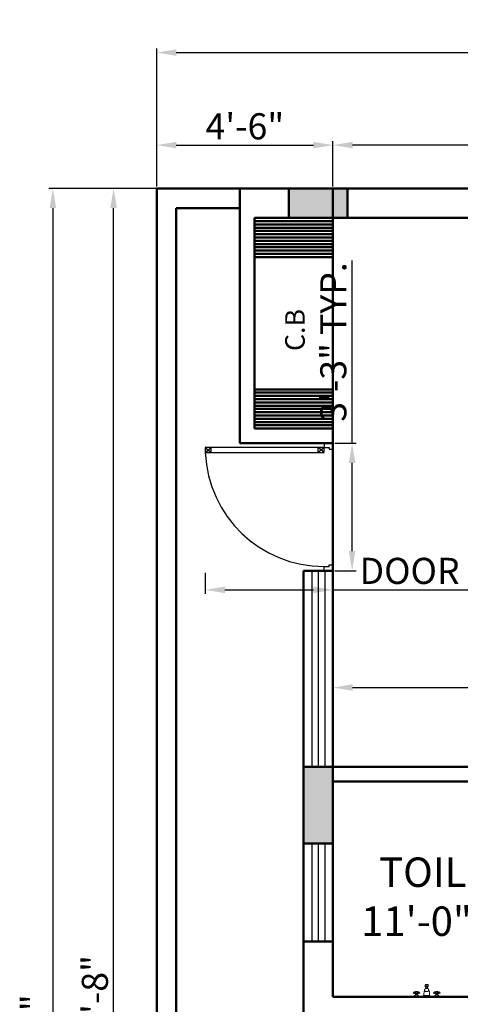
# Model space of a CAD drawing. Units: millimetres. Extents: x 1706 to 5913, y 156 to 1716.
# Tile 14 of 26: x 3136 to 3271, y 1414 to 1716. Entities that reach past the tile are written whole.
import ezdxf

# ---------------------------------------------------------------- set-up
doc = ezdxf.new("R2010")
doc.units = ezdxf.units.MM
for name, color, linetype, lineweight in [('A-ANNO-DIMS', 2, 'Continuous', 18), ('A-AREA-IDEN', 3, 'Continuous', 18), ('A-COLS', 20, 'Continuous', 50), ('A-DOOR', 4, 'Continuous', 25), ('A-FLOR-FIXT', 8, 'Continuous', 18), ('A-GLAZ', 150, 'Continuous', 25), ('A-WALL', 7, 'Continuous', 50)]:
    doc.layers.add(name, color=color, linetype=linetype, lineweight=lineweight)
doc.styles.get("Standard").update_dxf_attribs({"font": 'arial.ttf'})
doc.dimstyles.new('ISO-25', dxfattribs={"dimtxt": 8, "dimasz": 6, "dimexe": 1.25, "dimexo": 0.625, "dimtad": 1, "dimdec": 0, "dimlunit": 3, "dimtxsty": 'Standard', "dimcen": 2.5, "dimadec": 0, "dimazin": 0, "dimtfac": 1, "dimtdec": 0, "dimtmove": 0, "dimatfit": 3, "dimfxl": 1, "dimarcsym": 0})

# ---------------------------------------------------------------- blocks, each defined once
blk = doc.blocks.new('Puerta 01')
for p, q in [((-0.7745, -0.0264), (-0.7368, -0.0584)), ((-0.7745, -0.0584), (-0.7368, -0.0264)), ((-0.7368, -0.0584), (-0.7368, -0.0264)), ((-0.028, -0.0584), (-0.0657, -0.0264)), ((-0.028, -0.0264), (-0.0657, -0.0584)), ((-0.0657, -0.0584), (-0.0657, -0.0264))]:
    blk.add_line(p, q)
for points in [[(-0.028, 0), (-0.028, -0.0264), (0.004, -0.0264), (0.004, -0.036), (0.028, -0.036), (0.028, 0)], [(-0.028, -0.0264), (-0.7745, -0.0264), (-0.7745, -0.0584), (-0.028, -0.0584)], [(0.004, -0.7736), (0.004, -0.764), (0.028, -0.764), (0.028, -0.8), (-0.028, -0.8), (-0.028, -0.7736)]]:
    blk.add_lwpolyline(points, close=True)
blk.add_arc((-0.028, -0.0264), 0.7472, 182.45453, 270)
blk = doc.blocks.new('Faucet - Bathroom front')
for p, q in [((-0.5, 4.25), (0.5, 4.25)), ((0.5, 3.75), (-0.5, 3.75)), ((-5, 0), (-2.25, 0)), ((-4.5087, 0.25), (-2.7408, 0.25)), ((-4, 1.625), (-4.25, 1.625)), ((-4, 1.375), (-4.25, 1.375)), ((-3.1442, 0.75), (-4.0979, 0.75)), ((-3.25, 1.625), (-3, 1.625)), ((-3.25, 1.375), (-3, 1.375)), ((-1.5, 0), (1.5, 0)), ((-1, 0.5), (1, 0.5)), ((-0.5, 3), (0.5, 3)), ((0.5, 2), (-0.5, 2)), ((-0.25, 3), (-0.25, 3.5)), ((0.25, 3.5), (0.25, 3)), ((2.25, 0), (5, 0)), ((2.7413, 0.25), (4.5092, 0.25)), ((3.25, 1.625), (3, 1.625)), ((3.25, 1.375), (3, 1.375)), ((4.1058, 0.75), (3.1521, 0.75)), ((4, 1.625), (4.25, 1.625)), ((4, 1.375), (4.25, 1.375))]:
    blk.add_line(p, q)
for points in [[(-0.5, 3.75), (-0.5, 4.25)], [(-0.25, 4.5), (0.25, 4.5)], [(0.5, 4.25), (0.5, 3.75)], [(0.25, 3.5), (-0.25, 3.5)]]:
    blk.add_lwpolyline(points)
for points in [[(-4, 1), (-4, 2), (-3.25, 2), (-3.25, 1)], [(3.25, 1), (3.25, 2), (4, 2), (4, 1)]]:
    blk.add_lwpolyline(points, close=True)
for centre in [(-4.5, 1.5), (-3.625, 1.5), (-2.75, 1.5), (2.75, 1.5), (3.625, 1.5), (4.5, 1.5)]:
    blk.add_circle(centre, 0.2795)
for centre, radius, start, end in [((-0.2575, 4.2575), 0.2426, 88.22243, 181.7776), ((-0.2575, 3.7425), 0.2426, 178.2224, 271.7776), ((0.2575, 4.2575), 0.2426, 358.2224, 91.77757), ((0.2575, 3.7425), 0.2426, 268.2224, 1.777565), ((-5.375, 1.375), 1.4252, 285.2551, 344.7449), ((-1.875, 1.375), 1.4252, 195.2551, 254.7449), ((-0.7962, -0.2038), 0.7327, 106.1502, 163.8498), ((3, 1), 4.0311, 150.2551, 187.125), ((0.6413, 2.5), 1.246, 156.3417, 203.6583), ((-3, 1), 4.0311, 352.875, 29.74488), ((-0.6413, 2.5), 1.246, 336.3417, 23.65835), ((0.7962, -0.2038), 0.7327, 16.1502, 73.84979), ((1.875, 1.375), 1.4252, 285.2551, 344.7449), ((5.375, 1.375), 1.4252, 195.2551, 254.7449)]:
    blk.add_arc(centre, radius, start, end)
blk = doc.blocks.new('*D48')
at = {"layer": 'A-ANNO-DIMS', "color": 0, "lineweight": -2, "transparency": 16777216}
for p, q in [((3231.71, 1527.55), (3231.71, 1510.16)), ((3512.21, 1527.55), (3512.21, 1510.16)), ((3237.71, 1511.41), (3506.21, 1511.41))]:
    blk.add_line(p, q, dxfattribs=at)
at = {"layer": 'A-ANNO-DIMS', "color": 0, "transparency": 16777216}
for points in [[(3237.71, 1512.41), (3237.71, 1510.41), (3231.71, 1511.41)], [(3506.21, 1512.41), (3506.21, 1510.41), (3512.21, 1511.41)]]:
    blk.add_solid(points, dxfattribs=at)
at = {"layer": 'Defpoints', "color": 0, "transparency": 16777216}
for p in [(3231.71, 1528.17), (3512.21, 1528.17), (3512.21, 1511.41)]:
    blk.add_point(p, dxfattribs=at)
at = {"layer": 'A-ANNO-DIMS', "color": 0, "transparency": 16777216, "insert": (3371.96, 1516.12), "char_height": 8, "attachment_point": 5}
blk.add_mtext('23\'-5"', dxfattribs=at)
blk = doc.blocks.new('*D106')
at = {"layer": 'A-ANNO-DIMS', "color": 0, "lineweight": -2, "transparency": 16777216}
for p, q in [((3177.08, 1664.18), (3144.63, 1664.18)), ((3145.88, 1658.18), (3145.88, 1146.68)), ((3177.08, 1140.68), (3144.63, 1140.68))]:
    blk.add_line(p, q, dxfattribs=at)
at = {"layer": 'A-ANNO-DIMS', "color": 0, "transparency": 16777216}
for points in [[(3144.88, 1658.18), (3146.88, 1658.18), (3145.88, 1664.18)], [(3144.88, 1146.68), (3146.88, 1146.68), (3145.88, 1140.68)]]:
    blk.add_solid(points, dxfattribs=at)
at = {"layer": 'Defpoints', "color": 0, "transparency": 16777216}
for p in [(3177.71, 1664.18), (3145.88, 1140.68), (3177.71, 1140.68)]:
    blk.add_point(p, dxfattribs=at)
at = {"layer": 'A-ANNO-DIMS', "color": 0, "transparency": 16777216, "insert": (3141.17, 1402.43), "char_height": 8, "attachment_point": 5, "rotation": 90}
blk.add_mtext('43\'-8"', dxfattribs=at)
blk = doc.blocks.new('*D107')
at = {"layer": 'A-ANNO-DIMS', "color": 0, "lineweight": -2, "transparency": 16777216}
for p, q in [((3202.58, 1664.18), (3163.24, 1664.18)), ((3164.49, 1170.68), (3164.49, 1658.18)), ((3202.58, 1164.68), (3163.24, 1164.68))]:
    blk.add_line(p, q, dxfattribs=at)
at = {"layer": 'A-ANNO-DIMS', "color": 0, "transparency": 16777216}
for points in [[(3163.49, 1658.18), (3165.49, 1658.18), (3164.49, 1664.18)], [(3163.49, 1170.68), (3165.49, 1170.68), (3164.49, 1164.68)]]:
    blk.add_solid(points, dxfattribs=at)
at = {"layer": 'Defpoints', "color": 0, "transparency": 16777216}
for p in [(3164.49, 1664.18), (3203.21, 1664.18), (3203.21, 1164.68)]:
    blk.add_point(p, dxfattribs=at)
at = {"layer": 'A-ANNO-DIMS', "color": 0, "transparency": 16777216, "insert": (3159.78, 1414.43), "char_height": 8, "attachment_point": 5, "rotation": 90}
blk.add_mtext('41\'-8"', dxfattribs=at)
blk = doc.blocks.new('*D108')
at = {"layer": 'A-ANNO-DIMS', "color": 0, "lineweight": -2, "transparency": 16777216}
for p, q in [((3177.71, 1664.81), (3177.71, 1678.72)), ((3183.71, 1677.47), (3225.71, 1677.47)), ((3231.71, 1664.81), (3231.71, 1678.72))]:
    blk.add_line(p, q, dxfattribs=at)
at = {"layer": 'A-ANNO-DIMS', "color": 0, "transparency": 16777216}
for points in [[(3183.71, 1678.47), (3183.71, 1676.47), (3177.71, 1677.47)], [(3225.71, 1678.47), (3225.71, 1676.47), (3231.71, 1677.47)]]:
    blk.add_solid(points, dxfattribs=at)
at = {"layer": 'Defpoints', "color": 0, "transparency": 16777216}
for p in [(3231.71, 1677.47), (3177.71, 1664.18), (3231.71, 1664.18)]:
    blk.add_point(p, dxfattribs=at)
at = {"layer": 'A-ANNO-DIMS', "color": 0, "transparency": 16777216, "insert": (3204.71, 1682.18), "char_height": 8, "attachment_point": 5}
blk.add_mtext('4\'-6"', dxfattribs=at)
blk = doc.blocks.new('*D109')
at = {"layer": 'A-ANNO-DIMS', "color": 0, "lineweight": -2, "transparency": 16777216}
for p, q in [((3231.71, 1664.81), (3231.71, 1678.72)), ((3927.82, 1677.47), (3237.71, 1677.47)), ((3933.82, 1664.81), (3933.82, 1678.72))]:
    blk.add_line(p, q, dxfattribs=at)
at = {"layer": 'A-ANNO-DIMS', "color": 0, "transparency": 16777216}
for points in [[(3237.71, 1678.47), (3237.71, 1676.47), (3231.71, 1677.47)], [(3927.82, 1678.47), (3927.82, 1676.47), (3933.82, 1677.47)]]:
    blk.add_solid(points, dxfattribs=at)
at = {"layer": 'Defpoints', "color": 0, "transparency": 16777216}
for p in [(3231.71, 1677.47), (3231.71, 1664.18), (3933.82, 1664.18)]:
    blk.add_point(p, dxfattribs=at)
at = {"layer": 'A-ANNO-DIMS', "color": 0, "transparency": 16777216, "insert": (3582.76, 1682.18), "char_height": 8, "attachment_point": 5}
blk.add_mtext('58\'-6"', dxfattribs=at)
blk = doc.blocks.new('*D111')
at = {"layer": 'A-ANNO-DIMS', "color": 0, "lineweight": -2, "transparency": 16777216}
for p, q in [((3177.71, 1664.81), (3177.71, 1707.03)), ((4073, 1664.81), (4073, 1707.03)), ((3183.71, 1705.78), (4067, 1705.78))]:
    blk.add_line(p, q, dxfattribs=at)
at = {"layer": 'A-ANNO-DIMS', "color": 0, "transparency": 16777216}
for points in [[(3183.71, 1706.78), (3183.71, 1704.78), (3177.71, 1705.78)], [(4067, 1706.78), (4067, 1704.78), (4073, 1705.78)]]:
    blk.add_solid(points, dxfattribs=at)
at = {"layer": 'Defpoints', "color": 0, "transparency": 16777216}
for p in [(4073, 1705.78), (3177.71, 1664.18), (4073, 1664.18)]:
    blk.add_point(p, dxfattribs=at)
at = {"layer": 'A-ANNO-DIMS', "color": 0, "transparency": 16777216, "insert": (3625.35, 1710.41), "char_height": 8, "attachment_point": 5}
blk.add_mtext('74\'-7"', dxfattribs=at)
blk = doc.blocks.new('*D211')
at = {"layer": 'A-ANNO-DIMS', "color": 0, "lineweight": -2, "transparency": 16777216}
for p, q in [((3192.58, 1546.56), (3192.58, 1540.06)), ((3231.71, 1546.56), (3231.71, 1540.06)), ((3198.58, 1541.31), (3225.71, 1541.31)), ((3231.71, 1541.31), (3323.96, 1541.31))]:
    blk.add_line(p, q, dxfattribs=at)
at = {"layer": 'A-ANNO-DIMS', "color": 0, "transparency": 16777216}
for points in [[(3198.58, 1542.31), (3198.58, 1540.31), (3192.58, 1541.31)], [(3225.71, 1542.31), (3225.71, 1540.31), (3231.71, 1541.31)]]:
    blk.add_solid(points, dxfattribs=at)
at = {"layer": 'Defpoints', "color": 0, "transparency": 16777216}
for p in [(3192.58, 1547.18), (3231.71, 1547.18), (3231.71, 1541.31)]:
    blk.add_point(p, dxfattribs=at)
at = {"layer": 'A-ANNO-DIMS', "color": 0, "transparency": 16777216, "insert": (3280.83, 1546.08), "char_height": 8, "attachment_point": 5}
blk.add_mtext('DOOR 3\'-3" TYP.', dxfattribs=at)
blk = doc.blocks.new('*D212')
at = {"layer": 'A-ANNO-DIMS', "color": 0, "lineweight": -2, "transparency": 16777216}
for p, q in [((3237.58, 1586.18), (3237.58, 1642.19)), ((3232.33, 1586.18), (3238.83, 1586.18)), ((3237.58, 1553.18), (3237.58, 1580.18)), ((3232.33, 1547.18), (3238.83, 1547.18))]:
    blk.add_line(p, q, dxfattribs=at)
at = {"layer": 'A-ANNO-DIMS', "color": 0, "transparency": 16777216}
for points in [[(3236.58, 1580.18), (3238.58, 1580.18), (3237.58, 1586.18)], [(3236.58, 1553.18), (3238.58, 1553.18), (3237.58, 1547.18)]]:
    blk.add_solid(points, dxfattribs=at)
at = {"layer": 'Defpoints', "color": 0, "transparency": 16777216}
for p in [(3231.71, 1586.18), (3237.58, 1586.18), (3231.71, 1547.18)]:
    blk.add_point(p, dxfattribs=at)
at = {"layer": 'A-ANNO-DIMS', "color": 0, "transparency": 16777216, "insert": (3232.86, 1617.18), "char_height": 8, "attachment_point": 5, "rotation": 90}
blk.add_mtext('3\'-3" TYP.', dxfattribs=at)

msp = doc.modelspace()

# ---------------------------------------------------------------- hatches: boundary and pattern name
at = {"layer": 'A-COLS'}
h = msp.add_hatch(color=256, dxfattribs=at)
h.dxf.hatch_style = 1
h.paths.add_polyline_path([(3236.21, 1664.18), (3218.21, 1664.18), (3218.21, 1655.18), (3236.21, 1655.18)])
h = msp.add_hatch(color=256, dxfattribs=at)
h.dxf.hatch_style = 1
h.paths.add_polyline_path([(3231.71, 1487.18), (3222.71, 1487.18), (3222.71, 1463.68), (3231.71, 1463.68)])

# ---------------------------------------------------------------- linework, layer by layer
msp.add_lwpolyline([(3236.43, 1664.18), (3218.21, 1664.18), (3218.21, 1655.18), (3236.21, 1655.18), (3236.21, 1664.18)], dxfattribs=at)
msp.add_lwpolyline([(3231.71, 1487.18), (3222.71, 1487.18), (3222.71, 1463.68), (3231.71, 1463.68)], close=True, dxfattribs=at)
at = {"layer": 'A-GLAZ'}
for p, q in [((3225.21, 1547.18), (3225.21, 1487.18)), ((3227.21, 1547.18), (3227.21, 1487.18)), ((3229.21, 1547.18), (3229.21, 1487.18)), ((3225.21, 1463.68), (3225.21, 1433.68)), ((3227.21, 1463.68), (3227.21, 1433.68)), ((3229.21, 1463.68), (3229.21, 1433.68))]:
    msp.add_line(p, q, dxfattribs=at)
for points in [[(3231.71, 1487.18), (3222.71, 1487.18), (3222.71, 1547.18), (3231.71, 1547.18)], [(3231.71, 1433.68), (3222.71, 1433.68), (3222.71, 1463.68), (3231.71, 1463.68)]]:
    msp.add_lwpolyline(points, close=True, dxfattribs=at)
at = {"layer": 'A-WALL'}
for p, q in [((3177.71, 1664.18), (3203.21, 1664.18)), ((3177.71, 1664.18), (3177.71, 1140.68)), ((3203.21, 1664.18), (3203.21, 1586.18)), ((3203.21, 1664.18), (4017.71, 1664.18)), ((3231.71, 1664.18), (3231.71, 1487.18)), ((3236.21, 1655.18), (3236.21, 1664.18)), ((3236.21, 1664.18), (3236.21, 1655.18)), ((3183.71, 1658.18), (3183.71, 1170.68)), ((3183.71, 1658.18), (3203.21, 1658.18)), ((3207.71, 1655.18), (3207.71, 1590.68)), ((3207.71, 1655.18), (3605.21, 1655.18)), ((3207.71, 1654.18), (3231.71, 1654.18)), ((3207.71, 1653.18), (3231.71, 1653.18)), ((3207.71, 1652.18), (3231.71, 1652.18)), ((3207.71, 1651.18), (3231.71, 1651.18)), ((3207.71, 1650.18), (3231.71, 1650.18)), ((3207.71, 1649.18), (3231.71, 1649.18)), ((3207.71, 1648.18), (3231.71, 1648.18)), ((3207.71, 1647.18), (3231.71, 1647.18)), ((3207.71, 1646.18), (3231.71, 1646.18)), ((3207.71, 1645.18), (3231.71, 1645.18)), ((3207.71, 1644.18), (3231.71, 1644.18)), ((3207.71, 1643.18), (3231.71, 1643.18)), ((3207.71, 1602.68), (3231.71, 1602.68)), ((3207.71, 1601.68), (3231.71, 1601.68)), ((3207.71, 1600.68), (3231.71, 1600.68)), ((3207.71, 1599.68), (3231.71, 1599.68)), ((3207.71, 1598.68), (3231.71, 1598.68)), ((3207.71, 1597.68), (3231.71, 1597.68)), ((3207.71, 1596.68), (3231.71, 1596.68)), ((3207.71, 1595.68), (3231.71, 1595.68)), ((3207.71, 1594.68), (3231.71, 1594.68)), ((3207.71, 1593.68), (3231.71, 1593.68)), ((3207.71, 1592.68), (3231.71, 1592.68)), ((3207.71, 1591.68), (3231.71, 1591.68)), ((3207.71, 1590.68), (3231.71, 1590.68)), ((3203.21, 1586.18), (3231.71, 1586.18)), ((3222.71, 1547.18), (3231.71, 1547.18)), ((3222.71, 1547.18), (3222.71, 1281.68)), ((3231.71, 1487.18), (3431.21, 1487.18)), ((3231.71, 1482.68), (3431.21, 1482.68)), ((3231.71, 1482.68), (3231.71, 1416.68)), ((3222.71, 1463.68), (3231.71, 1463.68)), ((3222.71, 1433.68), (3231.71, 1433.68)), ((3231.71, 1416.68), (3363.71, 1416.68))]:
    msp.add_line(p, q, dxfattribs=at)

# ---------------------------------------------------------------- block references
at = {"layer": 'A-DOOR', "xscale": 48.75000000000287, "yscale": 48.75000000000287, "zscale": 48.75000000000287}
msp.add_blockref('Puerta 01', (3230.34, 1586.18), dxfattribs=at)
at = {"layer": 'A-FLOR-FIXT', "xscale": 0.8570205523683982, "yscale": 0.8570205523683982, "zscale": 0.8570205523683982}
msp.add_blockref('Faucet - Bathroom front', (3260.43, 1416.68), dxfattribs=at)

# ---------------------------------------------------------------- texts
at = {"layer": 'A-AREA-IDEN', "insert": (3217.07, 1605.26), "char_height": 6, "attachment_point": 1, "rotation": 90}
msp.add_mtext_dynamic_manual_height_columns('     C.B', width=33.9892, gutter_width=12.5, heights=[0], dxfattribs=at)
at = {"layer": 'A-AREA-IDEN', "insert": (3234.85, 1459.38), "char_height": 9, "attachment_point": 1}
msp.add_mtext_dynamic_manual_height_columns('    TOILET\\P  11\'-0"X5\'-6"', width=90.4844, gutter_width=12.5, heights=[0], dxfattribs=at)

# ---------------------------------------------------------------- dimensions: what is measured, and where the dimension line sits
at = {"layer": 'A-ANNO-DIMS'}
for base, p1, p2, picture, middle in [((4073, 1705.78), (3177.71, 1664.18), (4073, 1664.18), '*D111', (3625.35, 1710.41)), ((3231.71, 1677.47), (3177.71, 1664.18), (3231.71, 1664.18), '*D108', (3204.71, 1682.18)), ((3231.71, 1677.47), (3933.82, 1664.18), (3231.71, 1664.18), '*D109', (3582.76, 1682.18)), ((3512.20687195, 1511.4081474), (3231.70687195, 1528.17377043), (3512.20687195, 1528.17377043), '*D48', (3371.95687195, 1516.12045982))]:
    dim = msp.add_linear_dim(base=base, p1=p1, p2=p2, dimstyle='ISO-25', override={"dimclrd": 0, "dimclre": 0, "dimclrt": 0}, dxfattribs=at)
    dim.commit()
    dim.dimension.update_dxf_attribs({"geometry": picture, "text_midpoint": middle})
for base, p1, p2, picture, middle in [((3145.8779011, 1140.68004162), (3177.70687195, 1664.18004162), (3177.70687195, 1140.68004162), '*D106', (3141.16558869, 1402.43004162)), ((3164.4917582, 1664.18004162), (3203.20687195, 1164.68004162), (3203.20687195, 1664.18004162), '*D107', (3159.7821743, 1414.43004162))]:
    dim = msp.add_linear_dim(base=base, p1=p1, p2=p2, angle=90, dimstyle='ISO-25', override={"dimclrd": 0, "dimclre": 0, "dimclrt": 0}, dxfattribs=at)
    dim.commit()
    dim.dimension.update_dxf_attribs({"geometry": picture, "text_midpoint": middle})
dim = msp.add_linear_dim(base=(3237.58, 1586.18), p1=(3231.71, 1547.18), p2=(3231.71, 1586.18), angle=90, text='<> TYP.', dimstyle='ISO-25', override={"dimdec": 1, "dimrnd": 0, "dimzin": 1, "dimlunit": 4, "dimfrac": 2}, dxfattribs=at)
dim.commit()
dim.dimension.update_dxf_attribs({"geometry": '*D212', "text_midpoint": (3232.86, 1617.18)})
dim = msp.add_linear_dim(base=(3231.71, 1541.31), p1=(3192.58, 1547.18), p2=(3231.71, 1547.18), text='DOOR <> TYP.', dimstyle='ISO-25', override={"dimdec": 1, "dimrnd": 0, "dimzin": 1, "dimlunit": 4, "dimfrac": 2}, dxfattribs=at)
dim.commit()
dim.dimension.update_dxf_attribs({"geometry": '*D211', "text_midpoint": (3280.83, 1546.08)})

doc.saveas('drawing.dxf')
